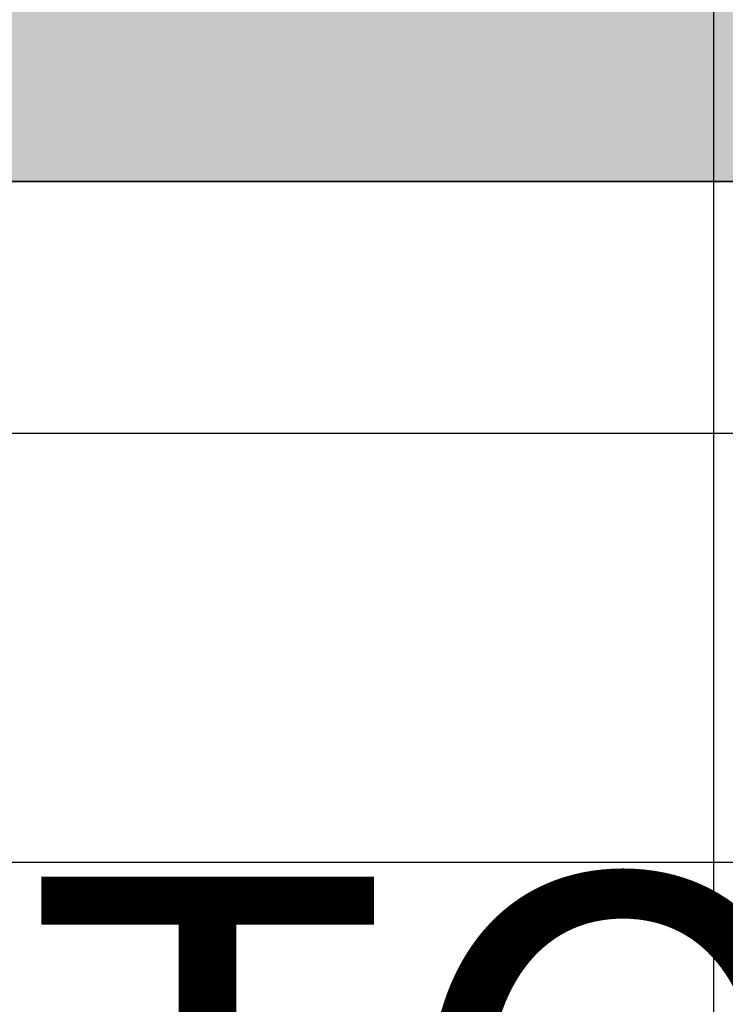
# Model space of a CAD drawing. Units: inches. Extents: x 2696 to 3240, y 1564 to 2310.
# Tile 17 of 76: x 2769 to 2783, y 1890 to 1910. Entities that reach past the tile are written whole.
import ezdxf

# ---------------------------------------------------------------- set-up
doc = ezdxf.new("R2010")
doc.units = ezdxf.units.IN
for name, color, linetype, lineweight in [('A-ANNO-DIMS', 3, 'Continuous', 18), ('A-AREA-IDEN', 7, 'Continuous', 18), ('A-WALL', 7, 'Continuous', 35), ('A-WALL-PATT', 9, 'Continuous', 13)]:
    doc.layers.add(name, color=color, linetype=linetype, lineweight=lineweight)
doc.styles.add('TIMES NEW', font='times.ttf')
doc.styles.add('YQ_DIM', font='SUPEROS.SHX', dxfattribs={"width": 0.8, "bigfont": 'HZDX.SHX'})
doc.dimstyles.new('Siddhuu', dxfattribs={"dimtxt": 6, "dimasz": 2.5, "dimexe": 1.25, "dimexo": 0.625, "dimtad": 1, "dimdec": 1, "dimlunit": 4, "dimtxsty": 'TIMES NEW', "dimcen": 2.5, "dimclrd": 256, "dimclre": 1, "dimclrt": 7, "dimadec": 0, "dimazin": 0, "dimtfac": 1, "dimtdec": 1, "dimtmove": 0, "dimatfit": 3, "dimfxl": 1, "dimtolj": 1, "dimlwd": -1, "dimarcsym": 0})

# ---------------------------------------------------------------- blocks, each defined once
blk = doc.blocks.new('*D55')
at = {"layer": 'A-ANNO-DIMS', "color": 1, "lineweight": -2, "transparency": 16777216}
for p, q in [((3189.986, 1980.201), (2709.361, 1980.201)), ((3189.986, 1893.201), (2709.361, 1893.201))]:
    blk.add_line(p, q, dxfattribs=at)
at = {"layer": 'A-ANNO-DIMS', "transparency": 16777216}
blk.add_line((2710.611, 1895.701), (2710.611, 1977.701), dxfattribs=at)
for points in [[(2710.195, 1977.701), (2711.028, 1977.701), (2710.611, 1980.201)], [(2710.195, 1895.701), (2711.028, 1895.701), (2710.611, 1893.201)]]:
    blk.add_solid(points, dxfattribs=at)
at = {"layer": 'Defpoints', "color": 0, "transparency": 16777216}
for p in [(2710.611, 1980.201), (3190.611, 1980.201), (3190.611, 1893.201)]:
    blk.add_point(p, dxfattribs=at)
at = {"layer": 'A-ANNO-DIMS', "color": 7, "transparency": 16777216, "insert": (2706.926, 1936.701), "char_height": 6, "attachment_point": 5, "rotation": 90, "style": 'TIMES NEW'}
blk.add_mtext('\\A1;7\'-3"', dxfattribs=at)
blk = doc.blocks.new('*D57')
at = {"layer": 'A-ANNO-DIMS', "color": 1, "lineweight": -2, "transparency": 16777216}
for p, q in [((2754.611, 2018.576), (2754.611, 1568.951)), ((2956.709, 2018.576), (2956.709, 1568.951))]:
    blk.add_line(p, q, dxfattribs=at)
at = {"layer": 'A-ANNO-DIMS', "transparency": 16777216}
blk.add_line((2757.111, 1570.201), (2954.209, 1570.201), dxfattribs=at)
for points in [[(2757.111, 1570.618), (2757.111, 1569.784), (2754.611, 1570.201)], [(2954.209, 1570.618), (2954.209, 1569.784), (2956.709, 1570.201)]]:
    blk.add_solid(points, dxfattribs=at)
at = {"layer": 'Defpoints', "color": 0, "transparency": 16777216}
for p in [(2754.611, 2019.201), (2956.709, 2019.201), (2956.709, 1570.201)]:
    blk.add_point(p, dxfattribs=at)
at = {"layer": 'A-ANNO-DIMS', "color": 7, "transparency": 16777216, "insert": (2855.66, 1573.878), "char_height": 6, "attachment_point": 5, "style": 'TIMES NEW'}
blk.add_mtext('\\A1;16\'-10"', dxfattribs=at)
blk = doc.blocks.new('*D68')
at = {"layer": 'A-ANNO-DIMS', "color": 1, "lineweight": -2, "transparency": 16777216}
for p, q in [((2745.611, 2261.576), (2745.611, 1568.951)), ((2782.834, 2261.576), (2782.834, 1568.951))]:
    blk.add_line(p, q, dxfattribs=at)
at = {"layer": 'A-ANNO-DIMS', "transparency": 16777216}
blk.add_line((2748.111, 1570.201), (2780.334, 1570.201), dxfattribs=at)
for points in [[(2748.111, 1570.618), (2748.111, 1569.784), (2745.611, 1570.201)], [(2780.334, 1570.618), (2780.334, 1569.784), (2782.834, 1570.201)]]:
    blk.add_solid(points, dxfattribs=at)
at = {"layer": 'Defpoints', "color": 0, "transparency": 16777216}
for p in [(2745.611, 2262.201), (2782.834, 2262.201), (2782.834, 1570.201)]:
    blk.add_point(p, dxfattribs=at)
at = {"layer": 'A-ANNO-DIMS', "color": 7, "transparency": 16777216, "insert": (2764.223, 1573.878), "char_height": 6, "attachment_point": 5, "style": 'TIMES NEW'}
blk.add_mtext('\\A1;3\'-1"', dxfattribs=at)
blk = doc.blocks.new('*D78')
at = {"layer": 'A-ANNO-DIMS', "transparency": 16777216}
for p, q in [((2710.611, 1901.701), (2710.611, 1935.101)), ((2710.611, 1895.701), (2710.611, 1899.201))]:
    blk.add_line(p, q, dxfattribs=at)
at = {"layer": 'A-ANNO-DIMS', "color": 1, "lineweight": -2, "transparency": 16777216}
for p, q in [((3189.986, 1901.701), (2709.361, 1901.701)), ((3189.986, 1893.201), (2709.361, 1893.201))]:
    blk.add_line(p, q, dxfattribs=at)
at = {"layer": 'A-ANNO-DIMS', "transparency": 16777216}
for points in [[(2710.195, 1899.201), (2711.028, 1899.201), (2710.611, 1901.701)], [(2710.195, 1895.701), (2711.028, 1895.701), (2710.611, 1893.201)]]:
    blk.add_solid(points, dxfattribs=at)
at = {"layer": 'Defpoints', "color": 0, "transparency": 16777216}
for p in [(2710.611, 1901.701), (3190.611, 1901.701), (3190.611, 1893.201)]:
    blk.add_point(p, dxfattribs=at)
at = {"layer": 'A-ANNO-DIMS', "color": 7, "transparency": 16777216, "insert": (2706.85, 1919.651), "char_height": 6, "attachment_point": 5, "rotation": 90, "style": 'TIMES NEW'}
blk.add_mtext('\\A1;0\'-8 1/2"', dxfattribs=at)

msp = doc.modelspace()

# ---------------------------------------------------------------- hatches: boundary and pattern name
at = {"layer": 'A-WALL-PATT', "transparency": 33554556}
h = msp.add_hatch(color=256, dxfattribs=at)
h.dxf.hatch_style = 1
h.paths.add_polyline_path([(2879.111, 2253.201), (2905.91, 2253.201), (2905.91, 2262.201), (2841.889, 2262.201), (2841.889, 2253.201), (2870.111, 2253.201), (2870.111, 2176.601), (2965.709, 2176.601), (2965.709, 2206.701), (2973.583, 2206.701), (2973.583, 2215.701), (2965.709, 2215.701), (2965.709, 2262.201), (2929.91, 2262.201), (2929.91, 2253.201), (2956.709, 2253.201), (2956.709, 2185.601), (2879.111, 2185.601)])
h.paths.add_polyline_path([(2782.834, 2262.201), (2745.611, 2262.201), (2745.611, 2228.729), (2754.611, 2228.729), (2754.611, 2253.201), (2782.834, 2253.201)])
h.paths.add_polyline_path([(2754.611, 2136.201), (2965.709, 2136.201), (2965.709, 2145.201), (2879.111, 2145.201), (2879.111, 2147.074), (2877.34, 2147.074), (2870.111, 2147.074), (2870.111, 2145.201), (2754.611, 2145.201), (2754.611, 2169.674), (2745.611, 2169.674), (2745.611, 2000.201), (2754.611, 2000.201), (2754.611, 2019.201), (2849.083, 2019.201), (2849.083, 2023.701), (2841.209, 2023.701), (2841.209, 2051.827), (2836.709, 2051.827), (2836.709, 2023.701), (2754.611, 2023.701), (2754.611, 2091.201), (2836.709, 2091.201), (2836.709, 2087.827), (2841.209, 2087.827), (2841.209, 2095.701), (2754.611, 2095.701)])
h.paths.add_polyline_path([(2965.709, 2136.201), (2956.709, 2136.201), (2956.709, 2023.701), (2885.083, 2023.701), (2885.083, 2019.201), (2956.709, 2019.201), (2956.709, 1950.575), (2965.709, 1950.575), (2965.709, 1980.201), (2973.583, 1980.201), (2973.583, 1989.201), (2965.709, 1989.201)])
h.paths.add_polyline_path([(2754.611, 1906.701), (2880.209, 1906.701), (2884.709, 1906.701), (2956.709, 1906.701), (2956.709, 1792.701), (2944.709, 1792.701), (2944.709, 1783.701), (2956.709, 1783.701), (2956.709, 1740.201), (2884.709, 1740.201), (2884.709, 1783.701), (2896.709, 1783.701), (2896.709, 1792.701), (2884.709, 1792.701), (2884.709, 1846.701), (2880.209, 1846.701), (2880.209, 1740.201), (2754.611, 1740.201), (2754.611, 1777.201), (2745.611, 1777.201), (2745.611, 1692.701), (2754.611, 1692.701), (2754.611, 1731.201), (2956.709, 1731.201), (2956.709, 1723.327), (2965.709, 1723.327), (2965.709, 1884.201), (2973.583, 1884.201), (2973.583, 1893.201), (2965.709, 1893.201), (2965.709, 1914.575), (2956.709, 1914.575), (2956.709, 1911.201), (2754.611, 1911.201), (2754.611, 1930.201), (2745.611, 1930.201), (2745.611, 1817.201), (2754.611, 1817.201), (2754.611, 1854.201), (2826.611, 1854.201), (2826.611, 1868.827), (2822.111, 1868.827), (2822.111, 1858.701), (2754.611, 1858.701)])
h.paths.add_polyline_path([(2965.709, 1656.201), (3008.237, 1656.201), (3008.237, 1665.201), (2965.709, 1665.201), (2965.709, 1693.327), (2956.709, 1693.327), (2956.709, 1686.201), (2934.583, 1686.201), (2934.583, 1681.701), (2956.709, 1681.701), (2956.709, 1614.201), (2896.709, 1614.201), (2896.709, 1681.701), (2904.583, 1681.701), (2904.583, 1686.201), (2892.209, 1686.201), (2892.209, 1614.201), (2858.41, 1614.201), (2858.41, 1605.201), (2965.709, 1605.201)])
h.paths.add_polyline_path([(2788.41, 1614.201), (2754.611, 1614.201), (2754.611, 1652.701), (2745.611, 1652.701), (2745.611, 1605.201), (2788.41, 1605.201)])
h.paths.add_polyline_path([(3199.611, 1633.048), (3190.611, 1633.048), (3190.611, 1614.201), (3082.611, 1614.201), (3082.611, 1665.201), (3070.237, 1665.201), (3070.237, 1656.201), (3078.111, 1656.201), (3078.111, 1605.201), (3199.611, 1605.201)])
h.paths.add_polyline_path([(3199.611, 1702.048), (3190.611, 1702.048), (3190.611, 1699.701), (3106.611, 1699.701), (3106.611, 1747.701), (3190.611, 1747.701), (3190.611, 1752.201), (3082.611, 1752.201), (3082.611, 1760.075), (3078.111, 1760.075), (3078.111, 1747.701), (3102.111, 1747.701), (3102.111, 1699.701), (3078.111, 1699.701), (3078.111, 1695.201), (3190.611, 1695.201), (3190.611, 1676.355), (3199.611, 1676.355)])
h.paths.add_polyline_path([(3199.611, 1783.201), (3190.611, 1783.201), (3190.611, 1745.355), (3199.611, 1745.355)])
h.paths.add_polyline_path([(3082.611, 1884.201), (3190.611, 1884.201), (3190.611, 1853.201), (3199.611, 1853.201), (3199.611, 1901.701), (3190.611, 1901.701), (3190.611, 1893.201), (3005.583, 1893.201), (3005.583, 1891.281), (3005.583, 1884.201), (3078.111, 1884.201), (3078.111, 1792.075), (3082.611, 1792.075)])
h.paths.add_polyline_path([(3199.611, 1994.701), (3190.611, 1994.701), (3190.611, 1989.201), (3073.709, 1989.201), (3073.709, 2034.201), (3069.209, 2034.201), (3069.209, 1989.201), (3005.583, 1989.201), (3005.583, 1980.201), (3190.611, 1980.201), (3190.611, 1971.701), (3199.611, 1971.701)])
h.paths.add_polyline_path([(3199.611, 2155.201), (3190.611, 2155.201), (3190.611, 2064.701), (3199.611, 2064.701)])
h.paths.add_polyline_path([(3190.611, 2074.701), (3106.611, 2074.701), (3106.611, 2122.701), (3190.611, 2122.701), (3190.611, 2127.201), (3082.709, 2127.201), (3082.709, 2135.075), (3073.709, 2135.075), (3073.709, 2122.701), (3102.111, 2122.701), (3102.111, 2074.701), (3069.209, 2074.701), (3069.209, 2070.201), (3190.611, 2070.201)])
h.paths.add_polyline_path([(3082.709, 2253.201), (3190.611, 2253.201), (3190.611, 2225.201), (3199.611, 2225.201), (3199.611, 2262.201), (3073.709, 2262.201), (3073.709, 2215.701), (3035.583, 2215.701), (3035.583, 2206.701), (3073.709, 2206.701), (3073.709, 2171.075), (3082.709, 2171.075)])

# ---------------------------------------------------------------- linework, layer by layer
at = {"layer": 'A-WALL'}
msp.add_line((2754.611, 1906.701), (2880.209, 1906.701), dxfattribs=at)

# ---------------------------------------------------------------- texts
at = {"layer": 'A-AREA-IDEN', "insert": (2769.129, 1892.921), "char_height": 9, "attachment_point": 1, "style": 'YQ_DIM'}
msp.add_mtext_dynamic_manual_height_columns('TOILET\\P5\'X5\'4.5"', width=48.00324, gutter_width=12.5, heights=[0], dxfattribs=at)

# ---------------------------------------------------------------- dimensions: what is measured, and where the dimension line sits
at = {"layer": 'A-ANNO-DIMS'}
for base, p1, p2, picture, middle in [((2782.834, 1570.201), (2745.611, 2262.201), (2782.834, 2262.201), '*D68', (2764.223, 1573.878)), ((2956.709, 1570.201), (2754.611, 2019.201), (2956.709, 2019.201), '*D57', (2855.66, 1573.878))]:
    dim = msp.add_linear_dim(base=base, p1=p1, p2=p2, dimstyle='Siddhuu', override={"dimdec": 1, "dimlfac": 1, "dimrnd": 0, "dimzin": 1, "dimdsep": 46, "dimlunit": 4, "dimfrac": 2}, dxfattribs=at)
    dim.commit()
    dim.dimension.update_dxf_attribs({"geometry": picture, "text_midpoint": middle})
for base, p2, picture, middle in [((2710.611, 1980.201), (3190.611, 1980.201), '*D55', (2706.926, 1936.701)), ((2710.611, 1901.701), (3190.611, 1901.701), '*D78', (2706.85, 1919.651))]:
    dim = msp.add_linear_dim(base=base, p1=(3190.611, 1893.201), p2=p2, angle=90, dimstyle='Siddhuu', override={"dimdec": 1, "dimlfac": 1, "dimrnd": 0, "dimzin": 1, "dimdsep": 46, "dimlunit": 4, "dimfrac": 2}, dxfattribs=at)
    dim.commit()
    dim.dimension.update_dxf_attribs({"geometry": picture, "text_midpoint": middle})

doc.saveas('drawing.dxf')
